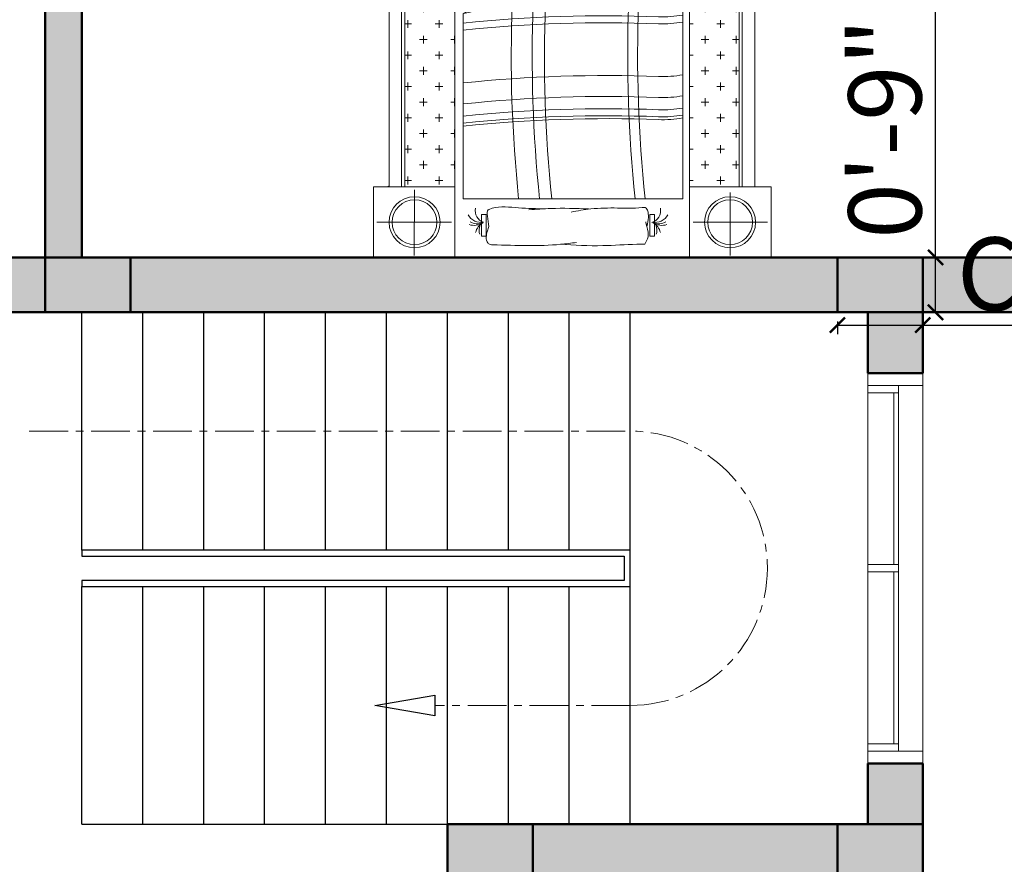
# Model space of a CAD drawing. Units: inches. Extents: x 375 to 1122, y 27 to 1069.
# Tile 81 of 155: x 784 to 945, y 577 to 716. Entities that reach past the tile are written whole.
import ezdxf

# ---------------------------------------------------------------- set-up
doc = ezdxf.new("R2010")
doc.units = ezdxf.units.IN
doc.linetypes.add('CENTER', pattern=[50.8, 31.75, -6.35, 6.35, -6.35])
for name, color, linetype, lineweight in [('A-ANNO-DIMS', 2, 'Continuous', 18), ('A-COLS-PATT', 10, 'Continuous', 13), ('A-FLOR-STRS-PATH', 40, 'CENTER', 18), ('A-WALL-PATT', 252, 'Continuous', 13), ('Columns', 10, 'Continuous', 50), ('Furniture', 30, 'Continuous', 18), ('Stairs', 40, 'Continuous', 25), ('Walls', 250, 'Continuous', 50), ('Windows', 122, 'Continuous', 18)]:
    doc.layers.add(name, color=color, linetype=linetype, lineweight=lineweight)
doc.styles.get("Standard").update_dxf_attribs({"font": 'arial.ttf'})
doc.dimstyles.new('ISO-25', dxfattribs={"dimtxt": 12, "dimasz": 2.5, "dimexe": 1.5, "dimexo": 1.5, "dimtad": 1, "dimdec": 1, "dimlunit": 3, "dimtxsty": 'Standard', "dimblk": 'ARCHTICK', "dimcen": 2.5, "dimadec": 0, "dimazin": 0, "dimtfac": 1, "dimtdec": 1, "dimtmove": 0, "dimatfit": 3, "dimfxl": 1.5, "dimfxlon": 1, "dimarcsym": 0})

# ---------------------------------------------------------------- blocks, each defined once
blk = doc.blocks.new('A$C52B64FF5')
for p, q in [((0.5216, 2.6276), (0, 2.6276)), ((0, 2.6276), (0, 2.1776)), ((0.2616, 2.4026), (0.2616, 2.6161)), ((0.5216, 2.1776), (0.5216, 2.6276)), ((2.0216, 2.6276), (0.5216, 2.6276)), ((0.5216, 2.6276), (0.5216, 0.6276)), ((2.5432, 2.6276), (2.0216, 2.6276)), ((2.0216, 0.6276), (2.0216, 2.6276)), ((2.0216, 2.6276), (2.0216, 2.1776)), ((2.2816, 2.4026), (2.2816, 2.6161)), ((2.5432, 2.1776), (2.5432, 2.6276)), ((0.721, 2.4927), (0.6917, 2.4927)), ((0.6917, 2.4927), (0.6917, 2.3531)), ((0.721, 2.3531), (0.721, 2.4927)), ((1.767, 2.3531), (1.767, 2.4927)), ((1.767, 2.4927), (1.7964, 2.4927)), ((1.7964, 2.4927), (1.7964, 2.3531)), ((0.2632, 2.4026), (0.0233, 2.4026)), ((0.0233, 2.4026), (0.4999, 2.4026)), ((0.2632, 2.1952), (0.2632, 2.4026)), ((2.5199, 2.4026), (2.0434, 2.4026)), ((2.2801, 2.2128), (2.2801, 2.4026)), ((2.2801, 2.4026), (2.5199, 2.4026)), ((0.6917, 2.3531), (0.721, 2.3531)), ((1.7964, 2.3531), (1.767, 2.3531)), ((0.5751, 1.0685), (0.5751, 2.2541)), ((0.5751, 2.2541), (1.9782, 2.2541)), ((1.9782, 2.2541), (1.9782, 0.6749)), ((0, 2.1776), (0.5216, 2.1776)), ((0.093, 2.1776), (0.1008, 2.1698)), ((0.1008, 0), (0.1008, 2.1776)), ((0.1808, 0.08), (0.1808, 2.1776)), ((0.2008, 0.1), (0.2008, 2.1776)), ((0.2197, 2.111), (0.2197, 2.161)), ((0.4197, 2.111), (0.4197, 2.161)), ((2.5432, 2.1776), (2.0216, 2.1776)), ((2.0216, 2.1776), (2.5432, 2.1776)), ((2.2197, 2.111), (2.2197, 2.161)), ((2.3374, 2.1776), (2.3374, 0.1)), ((2.3574, 2.1776), (2.3574, 0.08)), ((2.4374, 2.1776), (2.4374, 0)), ((0.2008, 2.136), (0.2447, 2.136)), ((0.3947, 2.136), (0.4447, 2.136)), ((2.0216, 2.136), (2.0447, 2.136)), ((2.1947, 2.136), (2.2447, 2.136)), ((0.2947, 2.036), (0.3447, 2.036)), ((0.3197, 2.011), (0.3197, 2.061)), ((0.4947, 2.036), (0.5216, 2.036)), ((0.5197, 2.011), (0.5197, 2.061)), ((2.0947, 2.036), (2.1447, 2.036)), ((2.1197, 2.011), (2.1197, 2.061)), ((2.2947, 2.036), (2.3374, 2.036)), ((2.3197, 2.011), (2.3197, 2.061)), ((0.2197, 1.911), (0.2197, 1.961)), ((0.4197, 1.911), (0.4197, 1.961)), ((2.2197, 1.911), (2.2197, 1.961)), ((0.2008, 1.936), (0.2447, 1.936)), ((0.3947, 1.936), (0.4447, 1.936)), ((2.0216, 1.936), (2.0447, 1.936)), ((2.1947, 1.936), (2.2447, 1.936)), ((0.2947, 1.836), (0.3447, 1.836)), ((0.3197, 1.811), (0.3197, 1.861)), ((0.4947, 1.836), (0.5216, 1.836)), ((0.5197, 1.811), (0.5197, 1.861)), ((2.0947, 1.836), (2.1447, 1.836)), ((2.1197, 1.811), (2.1197, 1.861)), ((2.2947, 1.836), (2.3374, 1.836)), ((2.3197, 1.811), (2.3197, 1.861)), ((0.2008, 1.736), (0.2447, 1.736)), ((0.2197, 1.711), (0.2197, 1.761)), ((0.3947, 1.736), (0.4447, 1.736)), ((0.4197, 1.711), (0.4197, 1.761)), ((2.0216, 1.736), (2.0447, 1.736)), ((2.1947, 1.736), (2.2447, 1.736)), ((2.2197, 1.711), (2.2197, 1.761)), ((0.3197, 1.611), (0.3197, 1.661)), ((0.5197, 1.611), (0.5197, 1.661)), ((2.1197, 1.611), (2.1197, 1.661)), ((2.3197, 1.611), (2.3197, 1.661)), ((0.2947, 1.636), (0.3447, 1.636)), ((0.4947, 1.636), (0.5216, 1.636)), ((2.0947, 1.636), (2.1447, 1.636)), ((2.2947, 1.636), (2.3374, 1.636)), ((0.2008, 1.536), (0.2447, 1.536)), ((0.2197, 1.511), (0.2197, 1.561)), ((0.3947, 1.536), (0.4447, 1.536)), ((0.4197, 1.511), (0.4197, 1.561)), ((2.0216, 1.536), (2.0447, 1.536)), ((2.1947, 1.536), (2.2447, 1.536)), ((2.2197, 1.511), (2.2197, 1.561)), ((0.3197, 1.411), (0.3197, 1.461)), ((0.5197, 1.411), (0.5197, 1.461)), ((2.1197, 1.411), (2.1197, 1.461)), ((2.3197, 1.411), (2.3197, 1.461)), ((0.2947, 1.436), (0.3447, 1.436)), ((0.4947, 1.436), (0.5216, 1.436)), ((2.0947, 1.436), (2.1447, 1.436)), ((2.2947, 1.436), (2.3374, 1.436)), ((0.2008, 1.336), (0.2447, 1.336)), ((0.2197, 1.311), (0.2197, 1.361)), ((0.3947, 1.336), (0.4447, 1.336)), ((0.4197, 1.311), (0.4197, 1.361)), ((2.0216, 1.336), (2.0447, 1.336)), ((2.1947, 1.336), (2.2447, 1.336)), ((2.2197, 1.311), (2.2197, 1.361)), ((0.3197, 1.211), (0.3197, 1.261)), ((0.5197, 1.211), (0.5197, 1.261)), ((2.1197, 1.211), (2.1197, 1.261)), ((2.3197, 1.211), (2.3197, 1.261)), ((0.2947, 1.236), (0.3447, 1.236)), ((0.4947, 1.236), (0.5216, 1.236)), ((2.0947, 1.236), (2.1447, 1.236)), ((2.2947, 1.236), (2.3374, 1.236)), ((0.2008, 1.136), (0.2447, 1.136)), ((0.2197, 1.111), (0.2197, 1.161)), ((0.3947, 1.136), (0.4447, 1.136)), ((0.4197, 1.111), (0.4197, 1.161)), ((2.0216, 1.136), (2.0447, 1.136)), ((2.1947, 1.136), (2.2447, 1.136)), ((2.2197, 1.111), (2.2197, 1.161)), ((0.2947, 1.036), (0.3447, 1.036)), ((0.3197, 1.011), (0.3197, 1.061)), ((0.4947, 1.036), (0.5216, 1.036)), ((0.5197, 1.011), (0.5197, 1.061)), ((2.0947, 1.036), (2.1447, 1.036)), ((2.1197, 1.011), (2.1197, 1.061)), ((2.2947, 1.036), (2.3374, 1.036)), ((2.3197, 1.011), (2.3197, 1.061)), ((0.2197, 0.911), (0.2197, 0.961)), ((0.4197, 0.911), (0.4197, 0.961)), ((2.2197, 0.911), (2.2197, 0.961)), ((2.4374, 0.9617), (2.4642, 0.935)), ((0.2008, 0.936), (0.2447, 0.936)), ((0.3947, 0.936), (0.4447, 0.936)), ((2.0216, 0.936), (2.0447, 0.936)), ((2.1947, 0.936), (2.2447, 0.936)), ((0.2947, 0.836), (0.3447, 0.836)), ((0.3197, 0.811), (0.3197, 0.861)), ((0.4947, 0.836), (0.5216, 0.836)), ((0.5197, 0.811), (0.5197, 0.861)), ((2.0947, 0.836), (2.1447, 0.836)), ((2.1197, 0.811), (2.1197, 0.861)), ((2.2947, 0.836), (2.3374, 0.836)), ((2.3197, 0.811), (2.3197, 0.861)), ((0.2197, 0.711), (0.2197, 0.761)), ((0.4197, 0.711), (0.4197, 0.761)), ((2.2197, 0.711), (2.2197, 0.761)), ((0.2008, 0.736), (0.2447, 0.736)), ((0.3947, 0.736), (0.4447, 0.736)), ((2.0216, 0.736), (2.0447, 0.736)), ((2.1947, 0.736), (2.2447, 0.736)), ((0.2947, 0.636), (0.3447, 0.636)), ((0.3197, 0.611), (0.3197, 0.661)), ((0.4947, 0.636), (0.5216, 0.636)), ((0.5197, 0.611), (0.5197, 0.661)), ((1.9782, 0.6749), (0.8764, 0.6749)), ((2.0947, 0.636), (2.1447, 0.636)), ((2.1197, 0.611), (2.1197, 0.661)), ((2.2947, 0.636), (2.3374, 0.636)), ((2.3197, 0.611), (2.3197, 0.661)), ((0.5216, 0.6276), (2.0216, 0.6276)), ((0.7197, 0.611), (0.7197, 0.6276)), ((0.9197, 0.611), (0.9197, 0.6276)), ((1.1197, 0.611), (1.1197, 0.6276)), ((1.3197, 0.611), (1.3197, 0.6276)), ((1.5197, 0.611), (1.5197, 0.6276)), ((1.7197, 0.611), (1.7197, 0.6276)), ((1.9197, 0.611), (1.9197, 0.6276)), ((0.2008, 0.536), (0.2447, 0.536)), ((0.2197, 0.511), (0.2197, 0.561)), ((0.3947, 0.536), (0.4447, 0.536)), ((0.4197, 0.511), (0.4197, 0.561)), ((0.5947, 0.536), (0.6447, 0.536)), ((0.6197, 0.511), (0.6197, 0.561)), ((0.7947, 0.536), (0.8447, 0.536)), ((0.8197, 0.511), (0.8197, 0.561)), ((0.9947, 0.536), (1.0447, 0.536)), ((1.0197, 0.511), (1.0197, 0.561)), ((1.1947, 0.536), (1.2447, 0.536)), ((1.2197, 0.511), (1.2197, 0.561)), ((1.3947, 0.536), (1.4447, 0.536)), ((1.4197, 0.511), (1.4197, 0.561)), ((1.5947, 0.536), (1.6447, 0.536)), ((1.6197, 0.511), (1.6197, 0.561)), ((1.7947, 0.536), (1.8447, 0.536)), ((1.8197, 0.511), (1.8197, 0.561)), ((1.9947, 0.536), (2.0447, 0.536)), ((2.0197, 0.511), (2.0197, 0.561)), ((2.1947, 0.536), (2.2447, 0.536)), ((2.2197, 0.511), (2.2197, 0.561)), ((0.3197, 0.411), (0.3197, 0.461)), ((0.5197, 0.411), (0.5197, 0.461)), ((0.7197, 0.411), (0.7197, 0.461)), ((0.9197, 0.411), (0.9197, 0.461)), ((1.1197, 0.411), (1.1197, 0.461)), ((1.3197, 0.411), (1.3197, 0.461)), ((1.5197, 0.411), (1.5197, 0.461)), ((1.7197, 0.411), (1.7197, 0.461)), ((1.9197, 0.411), (1.9197, 0.461)), ((2.1197, 0.411), (2.1197, 0.461)), ((2.3197, 0.411), (2.3197, 0.461)), ((0.2947, 0.436), (0.3447, 0.436)), ((0.4947, 0.436), (0.5447, 0.436)), ((0.6947, 0.436), (0.7447, 0.436)), ((0.8947, 0.436), (0.9447, 0.436)), ((1.0947, 0.436), (1.1447, 0.436)), ((1.2947, 0.436), (1.3447, 0.436)), ((1.4947, 0.436), (1.5447, 0.436)), ((1.6947, 0.436), (1.7447, 0.436)), ((1.8947, 0.436), (1.9447, 0.436)), ((2.0947, 0.436), (2.1447, 0.436)), ((2.2947, 0.436), (2.3374, 0.436)), ((0.2008, 0.336), (0.2447, 0.336)), ((0.2197, 0.311), (0.2197, 0.361)), ((0.3947, 0.336), (0.4447, 0.336)), ((0.4197, 0.311), (0.4197, 0.361)), ((0.5947, 0.336), (0.6447, 0.336)), ((0.6197, 0.311), (0.6197, 0.361)), ((0.7947, 0.336), (0.8447, 0.336)), ((0.8197, 0.311), (0.8197, 0.361)), ((0.9947, 0.336), (1.0447, 0.336)), ((1.0197, 0.311), (1.0197, 0.361)), ((1.1947, 0.336), (1.2447, 0.336)), ((1.2197, 0.311), (1.2197, 0.361)), ((1.3947, 0.336), (1.4447, 0.336)), ((1.4197, 0.311), (1.4197, 0.361)), ((1.5947, 0.336), (1.6447, 0.336)), ((1.6197, 0.311), (1.6197, 0.361)), ((1.7947, 0.336), (1.8447, 0.336)), ((1.8197, 0.311), (1.8197, 0.361)), ((1.9947, 0.336), (2.0447, 0.336)), ((2.0197, 0.311), (2.0197, 0.361)), ((2.1947, 0.336), (2.2447, 0.336)), ((2.2197, 0.311), (2.2197, 0.361)), ((0.3197, 0.211), (0.3197, 0.261)), ((0.5197, 0.211), (0.5197, 0.261)), ((0.7197, 0.211), (0.7197, 0.261)), ((0.9197, 0.211), (0.9197, 0.261)), ((1.1197, 0.211), (1.1197, 0.261)), ((1.3197, 0.211), (1.3197, 0.261)), ((1.5197, 0.211), (1.5197, 0.261)), ((1.7197, 0.211), (1.7197, 0.261)), ((1.9197, 0.211), (1.9197, 0.261)), ((2.1197, 0.211), (2.1197, 0.261)), ((2.3197, 0.211), (2.3197, 0.261)), ((0.2947, 0.236), (0.3447, 0.236)), ((0.4947, 0.236), (0.5447, 0.236)), ((0.6947, 0.236), (0.7447, 0.236)), ((0.8947, 0.236), (0.9447, 0.236)), ((1.0947, 0.236), (1.1447, 0.236)), ((1.2947, 0.236), (1.3447, 0.236)), ((1.4947, 0.236), (1.5447, 0.236)), ((1.6947, 0.236), (1.7447, 0.236)), ((1.8947, 0.236), (1.9447, 0.236)), ((2.0947, 0.236), (2.1447, 0.236)), ((2.2947, 0.236), (2.3374, 0.236)), ((0.2008, 0.136), (0.2447, 0.136)), ((0.2197, 0.111), (0.2197, 0.161)), ((0.3947, 0.136), (0.4447, 0.136)), ((0.4197, 0.111), (0.4197, 0.161)), ((0.5947, 0.136), (0.6447, 0.136)), ((0.6197, 0.111), (0.6197, 0.161)), ((0.7947, 0.136), (0.8447, 0.136)), ((0.8197, 0.111), (0.8197, 0.161)), ((0.9947, 0.136), (1.0447, 0.136)), ((1.0197, 0.111), (1.0197, 0.161)), ((1.1947, 0.136), (1.2447, 0.136)), ((1.2197, 0.111), (1.2197, 0.161)), ((1.3947, 0.136), (1.4447, 0.136)), ((1.4197, 0.111), (1.4197, 0.161)), ((1.5947, 0.136), (1.6447, 0.136)), ((1.6197, 0.111), (1.6197, 0.161)), ((1.7947, 0.136), (1.8447, 0.136)), ((1.8197, 0.111), (1.8197, 0.161)), ((1.9947, 0.136), (2.0447, 0.136)), ((2.0197, 0.111), (2.0197, 0.161)), ((2.1947, 0.136), (2.2447, 0.136)), ((2.2197, 0.111), (2.2197, 0.161)), ((2.3574, 0.08), (0.1808, 0.08)), ((2.3374, 0.1), (0.2008, 0.1)), ((2.4374, 0), (0.1008, 0))]:
    blk.add_line(p, q)
for centre, radius in [((0.2632, 2.4026), 0.1631), ((0.2632, 2.4026), 0.1431), ((2.2801, 2.4026), 0.1631), ((2.2801, 2.4026), 0.1431)]:
    blk.add_circle(centre, radius)
for centre, radius, start, end in [((0.7523, 2.4916), 0.1013, 192.77399, 239.2386), ((0.7566, 2.4523), 0.0808, 161.45592, 221.5545), ((1.7358, 2.4916), 0.1013, 300.7614, 347.22601), ((1.7315, 2.4523), 0.0808, 318.4455, 18.54408), ((0.6895, 2.3063), 0.098, 80.94857, 149.48786), ((0.6442, 2.3154), 0.1072, 59.2174, 107.24009), ((0.6646, 2.3215), 0.0913, 67.83977, 120.48585), ((0.7294, 2.33), 0.0776, 109.26419, 192.26691), ((1.7587, 2.33), 0.0776, 347.73309, 73.88358), ((1.7986, 2.3063), 0.098, 30.51214, 99.05143), ((1.8439, 2.3154), 0.1072, 72.75991, 120.7826), ((1.8235, 2.3215), 0.0913, 59.51415, 112.16023), ((9.7293, 1.3409), 8.8479, 174.07538, 182.16616), ((9.8633, 1.3409), 8.8479, 174.07538, 182.16616), ((9.9414, 1.3409), 8.8479, 174.07538, 182.16616), ((10.4736, 1.3409), 8.8479, 174.07538, 182.16616), ((10.5369, 1.3409), 8.8479, 174.07538, 182.16616), ((1.4884, 10.5889), 8.8479, 264.07538, 272.16616), ((1.4884, 10.5702), 8.8479, 264.07538, 272.16616), ((1.4884, 10.5256), 8.8479, 264.07538, 272.16616), ((1.85, 1.0282), 0.7196, 79.7409, 92.16616), ((1.85, 1.0096), 0.7196, 79.7409, 92.16616), ((1.4884, 10.4474), 8.8479, 264.07538, 272.16616), ((1.85, 0.965), 0.7196, 79.7409, 92.16616), ((1.85, 0.8868), 0.7196, 79.7409, 92.16616), ((1.4884, 10.3135), 8.8479, 264.07538, 272.16616), ((1.85, 0.7528), 0.7196, 79.7409, 92.16616), ((1.4884, 9.9764), 8.8479, 264.07538, 272.16616), ((1.85, 0.4158), 0.7196, 79.7409, 92.16616), ((1.4884, 9.9317), 8.8479, 264.07538, 272.16616), ((1.85, 0.3711), 0.7196, 79.7409, 92.16616), ((0.4865, 0.8516), 0.2343, 358.03681, 67.7864), ((0.5391, 0.7288), 0.3416, 350.92672, 83.95649), ((1.4884, 9.8536), 8.8479, 264.70583, 272.16616), ((1.85, 0.293), 0.7196, 79.7409, 92.16616), ((0.1687, 0.9792), 0.7196, 346.86533, 2.16616), ((0.3027, 0.9792), 0.7196, 334.98359, 2.16616), ((0.3808, 0.9792), 0.7196, 334.98359, 2.16616), ((0.913, 0.9792), 0.7196, 334.98359, 2.16616), ((0.9763, 0.9792), 0.7196, 334.98359, 2.16616), ((1.4884, 9.7196), 8.8479, 265.77852, 272.16616), ((0.5285, 0.5098), 0.3852, 25.3912, 60.06861), ((1.85, 0.159), 0.7196, 79.7409, 92.16616)]:
    blk.add_arc(centre, radius, start, end)
for points, knots in [([(0.7373, 2.4293), (0.7344, 2.4386), (0.7239, 2.472), (0.715, 2.518), (0.7414, 2.5459), (0.9088, 2.5514), (1.0864, 2.5586), (1.2642, 2.5365), (1.2976, 2.5323)], [0, 0, 0, 0, 0.0298664, 0.1071619, 0.1152509, 0.1416099, 0.5761797, 0.6768951, 0.6768951, 0.6768951, 0.6768951]), ([(1.1947, 2.5438), (1.2853, 2.549), (1.4483, 2.5585), (1.6283, 2.5432), (1.7179, 2.5437), (1.7351, 2.5438)], [0, 0, 0, 0, 0.2717358, 0.4891854, 0.5406465, 0.5406465, 0.5406465, 0.5406465]), ([(1.7351, 2.5438), (1.7416, 2.5321), (1.759, 2.5014), (1.7583, 2.4623), (1.7348, 2.3817), (1.7455, 2.4145), (1.7494, 2.4265)], [0, 0, 0, 0, 0.0383771, 0.1013156, 0.1484959, 0.1756343, 0.1756343, 0.1756343, 0.1756343]), ([(1.0802, 2.3175), (1.0225, 2.3155), (0.9099, 2.3116), (0.7905, 2.2985), (0.7234, 2.3279), (0.7309, 2.3766), (0.7348, 2.4091), (0.7373, 2.4293)], [0, 0, 0, 0, 0.1744349, 0.3406483, 0.347042, 0.3874998, 0.4538558, 0.4538558, 0.4538558, 0.4538558]), ([(1.7494, 2.4265), (1.7531, 2.4084), (1.7601, 2.3751), (1.7573, 2.3363), (1.7437, 2.3065), (1.6676, 2.315), (1.559, 2.3108), (1.4028, 2.3119), (1.305, 2.3301), (1.2633, 2.3378)], [0, 0, 0, 0, 0.0550284, 0.1011576, 0.1178362, 0.1437253, 0.3009935, 0.4726259, 0.6000038, 0.6000038, 0.6000038, 0.6000038]), ([(1.3748, 2.3178), (1.2947, 2.315), (1.1678, 2.3105), (1.0413, 2.32), (0.9946, 2.3235)], [0, 0, 0, 0, 0.2401688, 0.38052, 0.38052, 0.38052, 0.38052])]:
    blk.add_open_spline(points, degree=3, knots=knots)
blk = doc.blocks.new('COLUMN-14X9IN')
blk.add_lwpolyline([(0, 0), (14, 0), (14, 9), (0, 9)], close=True)
blk = doc.blocks.new('_ArchTick')
at = {"color": 0, "linetype": 'ByBlock', "const_width": 0.15}
blk.add_lwpolyline([(-0.5, -0.5), (0.5, 0.5)], dxfattribs=at)
blk = doc.blocks.new('*D41')
at = {"layer": 'A-ANNO-DIMS', "color": 0, "lineweight": -2, "transparency": 16777216}
for p, q in [((918.01, 666.03), (918.01, 663.93)), ((932.01, 666.03), (932.01, 663.93)), ((918.01, 665.43), (932.01, 665.43)), ((932.01, 665.43), (1086.07, 665.43))]:
    blk.add_line(p, q, dxfattribs=at)
at = {"layer": 'Defpoints', "color": 0, "transparency": 16777216}
for p in [(918.01, 667.53), (932.01, 667.53), (932.01, 665.43)]:
    blk.add_point(p, dxfattribs=at)
at = {"layer": 'A-ANNO-DIMS', "color": 0, "lineweight": -2, "transparency": 16777216, "xscale": 2.5, "yscale": 2.5, "zscale": 2.5, "rotation": 180}
blk.add_blockref('_ArchTick', (918.01, 665.43), dxfattribs=at)
at = {"layer": 'A-ANNO-DIMS', "color": 0, "lineweight": -2, "transparency": 16777216, "xscale": 2.5, "yscale": 2.5, "zscale": 2.5}
blk.add_blockref('_ArchTick', (932.01, 665.43), dxfattribs=at)
at = {"layer": 'A-ANNO-DIMS', "color": 0, "transparency": 16777216, "insert": (1010.29, 672.26), "char_height": 12, "attachment_point": 5}
blk.add_mtext('COLUMN 1\'-2" TYP.', dxfattribs=at)
blk = doc.blocks.new('*D42')
at = {"layer": 'A-ANNO-DIMS', "color": 0, "lineweight": -2, "transparency": 16777216}
for p, q in [((934.11, 676.53), (934.11, 753.42)), ((933.51, 676.53), (935.61, 676.53)), ((934.11, 667.53), (934.11, 676.53)), ((933.51, 667.53), (935.61, 667.53))]:
    blk.add_line(p, q, dxfattribs=at)
at = {"layer": 'Defpoints', "color": 0, "transparency": 16777216}
for p in [(932.01, 676.53), (934.11, 676.53), (932.01, 667.53)]:
    blk.add_point(p, dxfattribs=at)
at = {"layer": 'A-ANNO-DIMS', "color": 0, "lineweight": -2, "transparency": 16777216, "xscale": 2.5, "yscale": 2.5, "zscale": 2.5}
for p, rotation in [((934.11, 676.53), 90), ((934.11, 667.53), 270)]:
    blk.add_blockref('_ArchTick', p, dxfattribs=dict(at, rotation=rotation))
at = {"layer": 'A-ANNO-DIMS', "color": 0, "transparency": 16777216, "insert": (927.36, 716.23), "char_height": 12, "attachment_point": 5, "rotation": 90}
blk.add_mtext('0\'-9" TYP.', dxfattribs=at)
blk = doc.blocks.new('*D57')
at = {"layer": 'A-ANNO-DIMS', "color": 0, "lineweight": -2, "transparency": 16777216}
for p, q in [((512.46, 733.49), (512.46, 730.49)), ((512.46, 731.99), (638.07, 731.99)), ((638.07, 733.49), (638.07, 730.49)), ((638.07, 731.99), (839.76, 731.99))]:
    blk.add_line(p, q, dxfattribs=at)
at = {"layer": 'Defpoints', "color": 0, "transparency": 16777216}
for p in [(512.46, 750.84), (638.07, 750.84), (638.07, 731.99)]:
    blk.add_point(p, dxfattribs=at)
at = {"layer": 'A-ANNO-DIMS', "color": 0, "lineweight": -2, "transparency": 16777216, "xscale": 2.5, "yscale": 2.5, "zscale": 2.5, "rotation": 180}
blk.add_blockref('_ArchTick', (512.46, 731.99), dxfattribs=at)
at = {"layer": 'A-ANNO-DIMS', "color": 0, "lineweight": -2, "transparency": 16777216, "xscale": 2.5, "yscale": 2.5, "zscale": 2.5}
blk.add_blockref('_ArchTick', (638.07, 731.99), dxfattribs=at)
at = {"layer": 'A-ANNO-DIMS', "color": 0, "transparency": 16777216, "insert": (740.16, 738.83), "char_height": 12, "attachment_point": 5}
blk.add_mtext('SOFA SET 10\'-5 1/2" TYP.', dxfattribs=at)
blk = doc.blocks.new('*D84')
at = {"layer": 'A-ANNO-DIMS', "color": 0, "lineweight": -2, "transparency": 16777216}
for p, q in [((845.01, 117.53), (845.01, 114.53)), ((950.01, 117.53), (950.01, 114.53)), ((845.01, 116.03), (950.01, 116.03))]:
    blk.add_line(p, q, dxfattribs=at)
at = {"layer": 'Defpoints', "color": 0, "transparency": 16777216}
for p in [(845.01, 814.53), (950.01, 814.53), (950.01, 116.03)]:
    blk.add_point(p, dxfattribs=at)
at = {"layer": 'A-ANNO-DIMS', "color": 0, "lineweight": -2, "transparency": 16777216, "xscale": 2.5, "yscale": 2.5, "zscale": 2.5, "rotation": 180}
blk.add_blockref('_ArchTick', (845.01, 116.03), dxfattribs=at)
at = {"layer": 'A-ANNO-DIMS', "color": 0, "lineweight": -2, "transparency": 16777216, "xscale": 2.5, "yscale": 2.5, "zscale": 2.5}
blk.add_blockref('_ArchTick', (950.01, 116.03), dxfattribs=at)
at = {"layer": 'A-ANNO-DIMS', "color": 0, "transparency": 16777216, "insert": (897.51, 122.78), "char_height": 12, "attachment_point": 5}
blk.add_mtext('8\'-9"', dxfattribs=at)
blk = doc.blocks.new('*D86')
at = {"layer": 'A-ANNO-DIMS', "color": 0, "lineweight": -2, "transparency": 16777216}
for p, q in [((1032.01, 622.53), (1035.01, 622.53)), ((1033.51, 583.53), (1033.51, 622.53)), ((1032.01, 583.53), (1035.01, 583.53))]:
    blk.add_line(p, q, dxfattribs=at)
at = {"layer": 'Defpoints', "color": 0, "transparency": 16777216}
for p in [(884.01, 622.53), (1033.51, 622.53), (884.01, 583.53)]:
    blk.add_point(p, dxfattribs=at)
at = {"layer": 'A-ANNO-DIMS', "color": 0, "lineweight": -2, "transparency": 16777216, "xscale": 2.5, "yscale": 2.5, "zscale": 2.5}
for p, rotation in [((1033.51, 622.53), 90), ((1033.51, 583.53), 270)]:
    blk.add_blockref('_ArchTick', p, dxfattribs=dict(at, rotation=rotation))
at = {"layer": 'A-ANNO-DIMS', "color": 0, "transparency": 16777216, "insert": (1026.75, 603.03), "char_height": 12, "attachment_point": 5, "rotation": 90}
blk.add_mtext('3\'-3"', dxfattribs=at)
blk = doc.blocks.new('*D87')
at = {"layer": 'A-ANNO-DIMS', "color": 0, "lineweight": -2, "transparency": 16777216}
for p, q in [((794.01, 117.53), (794.01, 114.53)), ((884.01, 117.53), (884.01, 114.53)), ((794.01, 116.03), (884.01, 116.03))]:
    blk.add_line(p, q, dxfattribs=at)
at = {"layer": 'Defpoints', "color": 0, "transparency": 16777216}
for p in [(794.01, 583.53), (884.01, 583.53), (884.01, 116.03)]:
    blk.add_point(p, dxfattribs=at)
at = {"layer": 'A-ANNO-DIMS', "color": 0, "lineweight": -2, "transparency": 16777216, "xscale": 2.5, "yscale": 2.5, "zscale": 2.5, "rotation": 180}
blk.add_blockref('_ArchTick', (794.01, 116.03), dxfattribs=at)
at = {"layer": 'A-ANNO-DIMS', "color": 0, "lineweight": -2, "transparency": 16777216, "xscale": 2.5, "yscale": 2.5, "zscale": 2.5}
blk.add_blockref('_ArchTick', (884.01, 116.03), dxfattribs=at)
at = {"layer": 'A-ANNO-DIMS', "color": 0, "transparency": 16777216, "insert": (839.01, 122.78), "char_height": 12, "attachment_point": 5}
blk.add_mtext('7\'-6"', dxfattribs=at)
blk = doc.blocks.new('*D88')
at = {"layer": 'A-ANNO-DIMS', "color": 0, "lineweight": -2, "transparency": 16777216}
for p, q in [((731.01, 1052.53), (731.01, 1055.53)), ((854.01, 1052.53), (854.01, 1055.53)), ((731.01, 1054.03), (854.01, 1054.03))]:
    blk.add_line(p, q, dxfattribs=at)
at = {"layer": 'Defpoints', "color": 0, "transparency": 16777216}
for p in [(854.01, 1054.03), (731.01, 502.53), (854.01, 502.53)]:
    blk.add_point(p, dxfattribs=at)
at = {"layer": 'A-ANNO-DIMS', "color": 0, "lineweight": -2, "transparency": 16777216, "xscale": 2.5, "yscale": 2.5, "zscale": 2.5, "rotation": 180}
blk.add_blockref('_ArchTick', (731.01, 1054.03), dxfattribs=at)
at = {"layer": 'A-ANNO-DIMS', "color": 0, "lineweight": -2, "transparency": 16777216, "xscale": 2.5, "yscale": 2.5, "zscale": 2.5}
blk.add_blockref('_ArchTick', (854.01, 1054.03), dxfattribs=at)
at = {"layer": 'A-ANNO-DIMS', "color": 0, "transparency": 16777216, "insert": (792.51, 1060.78), "char_height": 12, "attachment_point": 5}
blk.add_mtext('10\'-3"', dxfattribs=at)

msp = doc.modelspace()

# ---------------------------------------------------------------- hatches: boundary and pattern name
at = {"layer": 'A-COLS-PATT'}
h = msp.add_hatch(color=256, dxfattribs=at)
h.dxf.hatch_style = 1
h.paths.add_polyline_path([(512.51, 982.53), (498.51, 982.53), (498.51, 973.53), (512.51, 973.53)])
h.paths.add_polyline_path([(666.51, 982.53), (652.51, 982.53), (652.51, 973.53), (666.51, 973.53)])
h.paths.add_polyline_path([(802.01, 982.53), (788.01, 982.53), (788.01, 973.53), (802.01, 973.53)])
h.paths.add_polyline_path([(932.01, 982.53), (918.01, 982.53), (918.01, 973.53), (932.01, 973.53)])
h.paths.add_polyline_path([(507.51, 841.53), (498.51, 841.53), (498.51, 827.53), (507.51, 827.53)])
h.paths.add_polyline_path([(666.51, 844.53), (652.51, 844.53), (652.51, 835.53), (666.51, 835.53)])
h.paths.add_polyline_path([(802.01, 814.53), (788.01, 814.53), (788.01, 805.53), (802.01, 805.53)])
h.paths.add_polyline_path([(932.01, 814.53), (918.01, 814.53), (918.01, 805.53), (932.01, 805.53)])
h.paths.add_polyline_path([(507.51, 719.53), (498.51, 719.53), (498.51, 705.53), (507.51, 705.53)])
h.paths.add_polyline_path([(731.01, 676.53), (722.01, 676.53), (722.01, 662.53), (731.01, 662.53)])
h.paths.add_polyline_path([(802.01, 676.53), (788.01, 676.53), (788.01, 667.53), (802.01, 667.53)])
h.paths.add_polyline_path([(932.01, 676.53), (918.01, 676.53), (918.01, 667.53), (932.01, 667.53)])
h.paths.add_polyline_path([(932.01, 583.53), (918.01, 583.53), (918.01, 574.53), (932.01, 574.53)])
h.paths.add_polyline_path([(868.01, 583.53), (854.01, 583.53), (854.01, 574.53), (868.01, 574.53)])
h.paths.add_polyline_path([(868.01, 502.53), (854.01, 502.53), (854.01, 493.53), (868.01, 493.53)])
h.paths.add_polyline_path([(932.01, 502.53), (918.01, 502.53), (918.01, 493.53), (932.01, 493.53)])
h.paths.add_polyline_path([(672.51, 592.03), (663.51, 592.03), (663.51, 578.03), (672.51, 578.03)])
h.paths.add_polyline_path([(512.51, 589.53), (498.51, 589.53), (498.51, 580.53), (512.51, 580.53)])
h.paths.add_polyline_path([(507.51, 464.53), (498.51, 464.53), (498.51, 450.53), (507.51, 450.53)])
h.paths.add_polyline_path([(731.01, 507.53), (722.01, 507.53), (722.01, 493.53), (731.01, 493.53)])
h.paths.add_polyline_path([(802.01, 502.53), (788.01, 502.53), (788.01, 493.53), (802.01, 493.53)])
h.paths.add_polyline_path([(507.51, 342.53), (498.51, 342.53), (498.51, 328.53), (507.51, 328.53)])
h.paths.add_polyline_path([(512.51, 196.53), (498.51, 196.53), (498.51, 187.53), (512.51, 187.53)])
h.paths.add_polyline_path([(666.51, 334.53), (652.51, 334.53), (652.51, 325.53), (666.51, 325.53)])
h.paths.add_polyline_path([(666.51, 196.53), (652.51, 196.53), (652.51, 187.53), (666.51, 187.53)])
h.paths.add_polyline_path([(805.01, 196.53), (791.01, 196.53), (791.01, 187.53), (805.01, 187.53)])
h.paths.add_polyline_path([(932.01, 196.53), (918.01, 196.53), (918.01, 187.53), (932.01, 187.53)])
h.paths.add_polyline_path([(932.01, 334.53), (918.01, 334.53), (918.01, 325.53), (932.01, 325.53)])
h.paths.add_polyline_path([(805.01, 334.53), (791.01, 334.53), (791.01, 325.53), (805.01, 325.53)])
at = {"layer": 'A-WALL-PATT'}
h = msp.add_hatch(color=256, dxfattribs=at)
h.dxf.hatch_style = 1
h.paths.add_polyline_path([(962.01, 388.53), (989.01, 388.53), (989.01, 394.53), (962.01, 394.53), (932.01, 394.53), (932.01, 397.53), (923.01, 397.53), (923.01, 394.53), (842.01, 394.53), (842.01, 334.53), (839.51, 334.53), (839.51, 328.53), (854.01, 328.53), (854.01, 334.53), (848.01, 334.53), (848.01, 388.53), (953.01, 388.53), (953.01, 356.08), (962.01, 356.08), (962.01, 358.55), (989.01, 358.55), (989.01, 364.55), (962.01, 364.55)])
h.paths.add_polyline_path([(989.01, 502.53), (932.01, 502.53), (932.01, 583.53), (932.01, 593.53), (923.01, 593.53), (923.01, 583.53), (854.01, 583.53), (854.01, 556.53), (863.01, 556.53), (863.01, 574.53), (923.01, 574.53), (923.01, 502.53), (863.01, 502.53), (863.01, 520.53), (854.01, 520.53), (854.01, 502.53), (773.01, 502.53), (773.01, 493.53), (788.01, 493.53), (788.01, 402.03), (722.01, 402.03), (722.01, 373.53), (728.01, 373.53), (728.01, 396.03), (788.01, 396.03), (788.01, 373.53), (794.01, 373.53), (794.01, 430.53), (814.01, 430.53), (814.01, 436.53), (794.01, 436.53), (794.01, 493.53), (923.01, 493.53), (923.01, 487.53), (932.01, 487.53), (932.01, 493.53), (983.01, 493.53), (983.01, 473.53), (989.01, 473.53)])
h.paths.add_polyline_path([(797.01, 325.53), (805.01, 325.53), (805.01, 328.53), (807.51, 328.53), (807.51, 334.53), (791.01, 334.53), (791.01, 226.53), (770.76, 226.53), (770.76, 217.53), (791.01, 217.53), (791.01, 187.53), (855.01, 187.53), (855.01, 196.53), (797.01, 196.53)])
h.paths.add_polyline_path([(989.01, 238.53), (962.01, 238.53), (962.01, 256.42), (953.01, 256.42), (953.01, 229.53), (980.01, 229.53), (980.01, 196.53), (915.01, 196.53), (915.01, 187.53), (989.01, 187.53)])
h.paths.add_polyline_path([(962.01, 334.53), (884.01, 334.53), (884.01, 328.53), (918.01, 328.53), (918.01, 325.53), (932.01, 325.53), (932.01, 328.53), (953.01, 328.53), (953.01, 304.42), (962.01, 304.42)])
h.paths.add_polyline_path([(606.51, 283.53), (609.51, 283.53), (609.51, 289.53), (600.51, 289.53), (600.51, 196.53), (578.51, 196.53), (578.51, 187.53), (606.51, 187.53), (606.51, 196.53)])
h.paths.add_polyline_path([(666.51, 292.53), (660.51, 292.53), (660.51, 289.53), (633.51, 289.53), (633.51, 283.53), (660.51, 283.53), (660.51, 196.53), (628.01, 196.53), (628.01, 187.53), (630.53, 187.53), (630.53, 160.53), (636.53, 160.53), (636.53, 187.53), (660.51, 187.53), (660.51, 160.53), (666.51, 160.53), (666.51, 217.53), (686.76, 217.53), (686.76, 226.53), (666.51, 226.53)])
h.paths.add_polyline_path([(480.51, 256.42), (471.51, 256.42), (471.51, 238.53), (444.51, 238.53), (444.51, 187.53), (518.51, 187.53), (518.51, 196.53), (453.51, 196.53), (453.51, 229.53), (480.51, 229.53)])
h.paths.add_polyline_path([(480.51, 328.53), (652.51, 328.53), (652.51, 325.53), (660.51, 325.53), (660.51, 322.53), (666.51, 322.53), (666.51, 334.53), (507.51, 334.53), (507.51, 360.53), (498.51, 360.53), (498.51, 334.53), (471.51, 334.53), (471.51, 304.42), (480.51, 304.42)])
h.paths.add_polyline_path([(507.51, 484.53), (498.51, 484.53), (498.51, 444.53), (507.51, 444.53), (507.51, 454.53), (621.51, 454.53), (621.51, 460.53), (507.51, 460.53)])
h.paths.add_polyline_path([(672.51, 604.53), (683.26, 604.53), (683.26, 613.53), (669.51, 613.53), (669.51, 649.53), (663.51, 649.53), (663.51, 589.53), (507.51, 589.53), (507.51, 613.53), (498.51, 613.53), (498.51, 556.53), (507.51, 556.53), (507.51, 580.53), (663.51, 580.53), (663.51, 520.53), (669.51, 520.53), (669.51, 556.53), (683.26, 556.53), (683.26, 565.53), (672.51, 565.53)])
h.paths.add_polyline_path([(731.01, 667.53), (734.01, 667.53), (734.01, 676.53), (728.01, 676.53), (728.01, 715.53), (657.51, 715.53), (657.51, 709.53), (663.51, 709.53), (663.51, 673.53), (669.51, 673.53), (669.51, 709.53), (722.01, 709.53), (722.01, 613.53), (704.76, 613.53), (704.76, 604.53), (722.01, 604.53), (722.01, 565.53), (704.76, 565.53), (704.76, 556.53), (722.01, 556.53), (722.01, 502.53), (722.01, 460.53), (669.51, 460.53), (669.51, 496.53), (663.51, 496.53), (663.51, 460.53), (657.51, 460.53), (657.51, 454.53), (728.01, 454.53), (728.01, 493.53), (734.01, 493.53), (734.01, 502.53), (731.01, 502.53)])
h.paths.add_polyline_path([(986.01, 718.53), (959.01, 718.53), (959.01, 727.53), (950.01, 727.53), (950.01, 709.53), (977.01, 709.53), (977.01, 676.53), (794.01, 676.53), (794.01, 805.53), (802.01, 805.53), (802.01, 808.53), (804.51, 808.53), (804.51, 814.53), (788.01, 814.53), (788.01, 774.03), (728.01, 774.03), (728.01, 796.53), (722.01, 796.53), (722.01, 768.03), (788.01, 768.03), (788.01, 676.53), (773.01, 676.53), (773.01, 667.53), (923.01, 667.53), (923.01, 657.53), (932.01, 657.53), (932.01, 667.53), (986.01, 667.53)])
h.paths.add_polyline_path([(621.51, 715.53), (507.51, 715.53), (507.51, 733.53), (498.51, 733.53), (498.51, 715.53), (498.51, 685.53), (507.51, 685.53), (507.51, 709.53), (621.51, 709.53)])
h.paths.add_polyline_path([(666.51, 847.03), (660.51, 847.03), (660.51, 844.53), (652.51, 844.53), (652.51, 841.53), (480.51, 841.53), (480.51, 859.53), (471.51, 859.53), (471.51, 835.53), (498.51, 835.53), (498.51, 817.53), (507.51, 817.53), (507.51, 835.53), (666.51, 835.53)])
h.paths.add_polyline_path([(480.51, 940.53), (453.51, 940.53), (453.51, 973.53), (518.51, 973.53), (518.51, 982.53), (444.51, 982.53), (444.51, 931.53), (471.51, 931.53), (471.51, 907.53), (480.51, 907.53)])
h.paths.add_polyline_path([(606.51, 982.53), (578.51, 982.53), (578.51, 973.53), (600.51, 973.53), (600.51, 880.53), (609.51, 880.53), (609.51, 886.53), (606.51, 886.53)])
h.paths.add_polyline_path([(666.51, 943.53), (686.76, 943.53), (686.76, 952.53), (666.51, 952.53), (666.51, 1009.53), (660.51, 1009.53), (660.51, 982.53), (636.53, 982.53), (636.53, 1009.53), (630.53, 1009.53), (630.53, 982.53), (628.01, 982.53), (628.01, 973.53), (660.51, 973.53), (660.51, 886.53), (633.51, 886.53), (633.51, 880.53), (660.51, 880.53), (660.51, 877.03), (666.51, 877.03)])
h.paths.add_polyline_path([(986.01, 874.53), (932.01, 874.53), (932.01, 877.53), (923.01, 877.53), (923.01, 874.53), (788.01, 874.53), (788.01, 868.53), (788.01, 844.53), (794.01, 844.53), (794.01, 868.53), (839.01, 868.53), (839.01, 814.53), (836.51, 814.53), (836.51, 808.53), (851.01, 808.53), (851.01, 814.53), (845.01, 814.53), (845.01, 868.53), (986.01, 868.53)])
h.paths.add_polyline_path([(959.01, 838.55), (986.01, 838.55), (986.01, 844.55), (959.01, 844.55), (959.01, 847.03), (950.01, 847.03), (950.01, 814.53), (881.01, 814.53), (881.01, 808.53), (918.01, 808.53), (918.01, 805.53), (932.01, 805.53), (932.01, 808.53), (950.01, 808.53), (950.01, 793.53), (959.01, 793.53)])
h.paths.add_polyline_path([(986.01, 982.53), (899.01, 982.53), (899.01, 973.53), (923.01, 973.53), (923.01, 967.53), (932.01, 967.53), (932.01, 973.53), (980.01, 973.53), (980.01, 953.53), (986.01, 953.53)])
h.paths.add_polyline_path([(851.01, 982.53), (788.01, 982.53), (788.01, 952.53), (770.76, 952.53), (770.76, 943.53), (788.01, 943.53), (788.01, 910.53), (814.01, 910.53), (814.01, 916.53), (794.01, 916.53), (794.01, 973.53), (851.01, 973.53)])

# ---------------------------------------------------------------- linework, layer by layer
at = {"layer": 'A-FLOR-STRS-PATH', "ltscale": 0.2}
msp.add_lwpolyline([(785.39, 648.03), (884.01, 648.03, -1), (884.01, 603.03), (851.96, 603.03)], format="xyb", dxfattribs=at)
at = {"layer": 'Stairs'}
for p, q in [((794.01, 628.53), (794.01, 667.53)), ((804.01, 628.53), (804.01, 667.53)), ((814.01, 628.53), (814.01, 667.53)), ((824.01, 628.53), (824.01, 667.53)), ((834.01, 628.53), (834.01, 667.53)), ((844.01, 628.53), (844.01, 667.53)), ((854.01, 628.53), (854.01, 667.53)), ((864.01, 628.53), (864.01, 667.53)), ((874.01, 628.53), (874.01, 667.53)), ((884.01, 628.53), (884.01, 667.53)), ((794.01, 583.53), (794.01, 622.53)), ((804.01, 583.53), (804.01, 622.53)), ((814.01, 583.53), (814.01, 622.53)), ((824.01, 583.53), (824.01, 622.53)), ((834.01, 583.53), (834.01, 622.53)), ((844.01, 583.53), (844.01, 622.53)), ((854.01, 583.53), (854.01, 622.53)), ((864.01, 583.53), (864.01, 622.53)), ((874.01, 583.53), (874.01, 622.53)), ((884.01, 583.53), (884.01, 622.53)), ((794.01, 583.53), (884.01, 583.53))]:
    msp.add_line(p, q, dxfattribs=at)
for points in [[(794.01, 622.53), (884.01, 622.53), (884.01, 628.53), (794.01, 628.53), (794.01, 627.53), (883.01, 627.53), (883.01, 623.53), (794.01, 623.53)], [(842.07, 603.03), (851.96, 604.7), (851.96, 601.35)]]:
    msp.add_lwpolyline(points, close=True, dxfattribs=at)
at = {"layer": 'Walls'}
for p, q in [((794.01, 805.53), (794.01, 676.53)), ((788.01, 768.03), (788.01, 676.53)), ((788.01, 676.53), (773.01, 676.53)), ((977.01, 676.53), (794.01, 676.53)), ((923.01, 667.53), (773.01, 667.53)), ((923.01, 657.53), (923.01, 667.53)), ((986.01, 667.53), (932.01, 667.53)), ((932.01, 657.53), (932.01, 667.53)), ((923.01, 657.53), (932.01, 657.53)), ((923.01, 583.53), (923.01, 593.53)), ((923.01, 593.53), (932.01, 593.53)), ((932.01, 583.53), (932.01, 593.53)), ((923.01, 583.53), (854.01, 583.53)), ((854.01, 556.53), (854.01, 583.53)), ((932.01, 502.53), (932.01, 583.53))]:
    msp.add_line(p, q, dxfattribs=at)
at = {"layer": 'Windows'}
for p, q in [((927.26, 654.33), (927.26, 626.13)), ((928.01, 654.33), (928.01, 596.73)), ((927.26, 624.93), (927.26, 596.73))]:
    msp.add_line(p, q, dxfattribs=at)
for points in [[(923.01, 657.53), (932.01, 657.53), (932.01, 593.53), (923.01, 593.53)], [(923.01, 654.33), (928.01, 654.33), (928.01, 655.53), (923.01, 655.53)], [(923.01, 624.93), (928.01, 624.93), (928.01, 626.13), (923.01, 626.13)], [(923.01, 596.73), (928.01, 596.73), (928.01, 595.53), (923.01, 595.53)]]:
    msp.add_lwpolyline(points, close=True, dxfattribs=at)
for points in [[(923.01, 655.53), (932.01, 655.53)], [(932.01, 595.53), (923.01, 595.53)]]:
    msp.add_lwpolyline(points, dxfattribs=at)

# ---------------------------------------------------------------- block references
at = {"layer": 'Columns'}
for p in [(788.01, 667.53), (918.01, 667.53), (918.01, 574.53)]:
    msp.add_blockref('COLUMN-14X9IN', p, dxfattribs=at)
at = {"layer": 'Columns', "extrusion": (0, 0, -1), "zscale": -1}
msp.add_blockref('COLUMN-14X9IN', (-868.01, 574.53), dxfattribs=at)
at = {"layer": 'Furniture', "xscale": -25.67804170018038, "yscale": 25.67804170018038, "zscale": 25.67804170018038, "rotation": 180}
msp.add_blockref('A$C52B64FF5', (841.85, 744), dxfattribs=at)

# ---------------------------------------------------------------- dimensions: what is measured, and where the dimension line sits
at = {"layer": 'A-ANNO-DIMS'}
for base, p1, p2, picture, middle in [((854.01, 1054.03), (731.01, 502.53), (854.01, 502.53), '*D88', (792.51, 1060.78)), ((950.01, 116.03), (845.01, 814.53), (950.01, 814.53), '*D84', (897.51, 122.78)), ((884.01, 116.03), (794.01, 583.53), (884.01, 583.53), '*D87', (839.01, 122.78))]:
    dim = msp.add_linear_dim(base=base, p1=p1, p2=p2, dimstyle='ISO-25', override={"dimdec": 1, "dimlfac": 1, "dimrnd": 0, "dimzin": 1, "dimdsep": 46, "dimlunit": 4, "dimfrac": 2}, dxfattribs=at)
    dim.commit()
    dim.dimension.update_dxf_attribs({"geometry": picture, "text_midpoint": middle})
for base, p1, p2, text, picture, middle in [((638.07, 731.99), (512.46, 750.84), (638.07, 750.84), 'SOFA SET <> TYP.', '*D57', (740.16, 738.83)), ((932.01, 665.43), (918.01, 667.53), (932.01, 667.53), 'COLUMN <> TYP.', '*D41', (1010.29, 672.26))]:
    dim = msp.add_linear_dim(base=base, p1=p1, p2=p2, text=text, dimstyle='ISO-25', override={"dimdec": 1, "dimlfac": 1, "dimrnd": 0, "dimzin": 1, "dimdsep": 46, "dimlunit": 4, "dimfrac": 2}, dxfattribs=at)
    dim.commit()
    dim.dimension.update_dxf_attribs({"geometry": picture, "text_midpoint": middle})
dim = msp.add_linear_dim(base=(934.11, 676.53), p1=(932.01, 667.53), p2=(932.01, 676.53), angle=90, text='<> TYP.', dimstyle='ISO-25', override={"dimdec": 1, "dimlfac": 1, "dimrnd": 0, "dimzin": 1, "dimdsep": 46, "dimlunit": 4, "dimfrac": 2}, dxfattribs=at)
dim.commit()
dim.dimension.update_dxf_attribs({"geometry": '*D42', "text_midpoint": (927.36, 716.23)})
dim = msp.add_linear_dim(base=(1033.51, 622.53), p1=(884.01, 583.53), p2=(884.01, 622.53), angle=90, dimstyle='ISO-25', override={"dimdec": 1, "dimlfac": 1, "dimrnd": 0, "dimzin": 1, "dimdsep": 46, "dimlunit": 4, "dimfrac": 2}, dxfattribs=at)
dim.commit()
dim.dimension.update_dxf_attribs({"geometry": '*D86', "text_midpoint": (1026.75, 603.03)})

doc.saveas('drawing.dxf')
